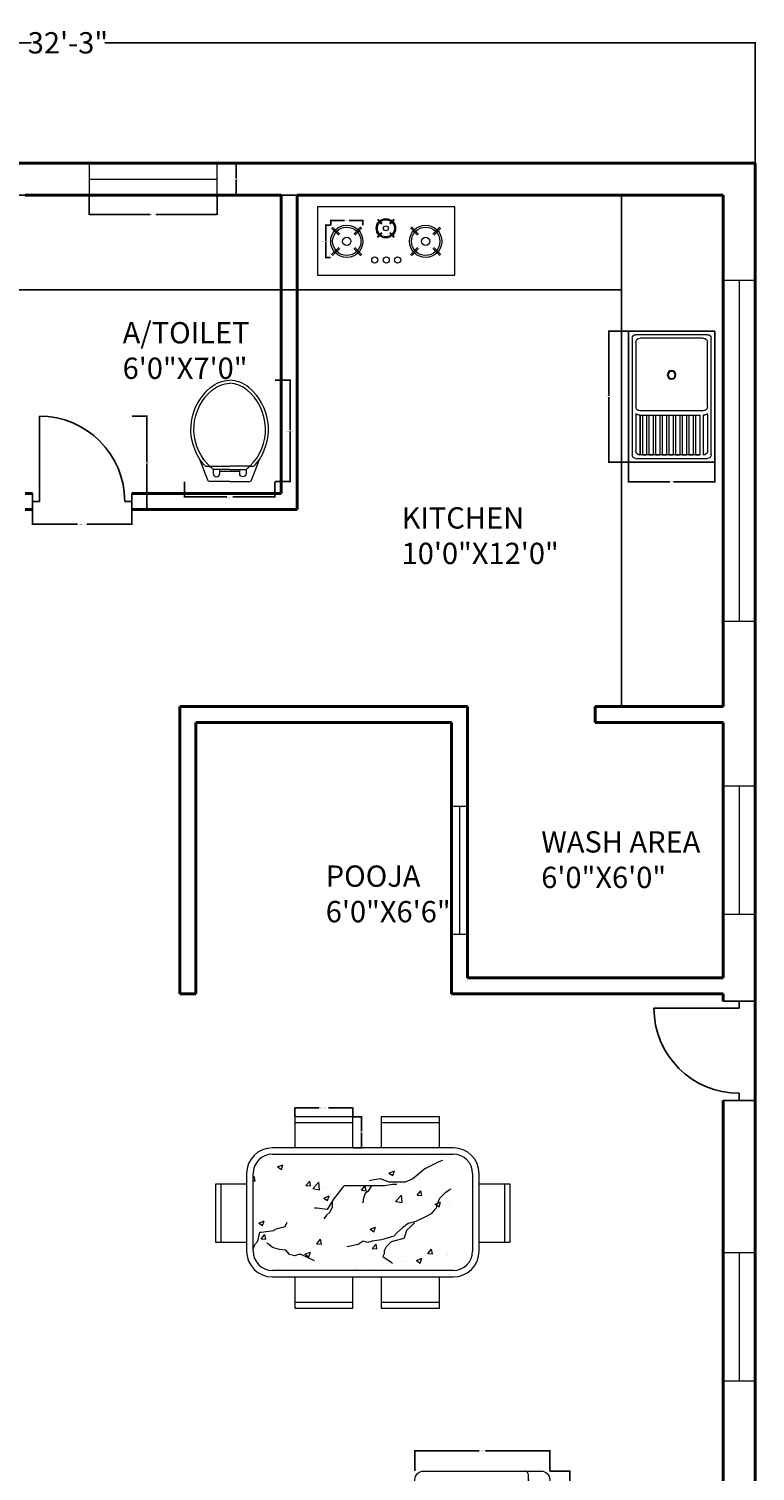
# Model space of a CAD drawing. Units: inches. Extents: x -19 to 419, y -828 to 43.
# Tile 9 of 9: x 205 to 410, y -364 to 43. Entities that reach past the tile are written whole.
import ezdxf

# ---------------------------------------------------------------- set-up
doc = ezdxf.new("R2010")
doc.units = ezdxf.units.IN
doc.header["$MEASUREMENT"] = 0
for name, color, linetype, lineweight in [('A-ANNO-DIMS', 2, 'Continuous', 18), ('A-AREA-IDEN', 7, 'Continuous', 25), ('A-DOOR', 3, 'Continuous', 25), ('A-EQPM', 9, 'Continuous', 20), ('A-FLOR-CASE', 8, 'Continuous', 25), ('A-FLOR-FIXT', 9, 'Continuous', 20), ('A-FURN', 8, 'Continuous', 18), ('A-FURN-PATT', 252, 'Continuous', 13), ('A-GLAZ', 4, 'Continuous', 20), ('A-WALL', 7, 'Continuous', 40)]:
    doc.layers.add(name, color=color, linetype=linetype, lineweight=lineweight)
doc.styles.get("Standard").update_dxf_attribs({"font": 'arial.ttf'})
doc.dimstyles.get("Standard").update_dxf_attribs({"dimtxt": 0.18, "dimasz": 0.18, "dimexe": 0.18, "dimexo": 0.0625, "dimgap": 0.09, "dimtad": 0, "dimtih": 1, "dimtoh": 1, "dimdec": 0, "dimzin": 0, "dimdsep": 46, "dimlunit": 3, "dimtxsty": 'Standard', "dimcen": 0.09, "dimadec": 0, "dimazin": 0, "dimtfac": 1, "dimtdec": 0, "dimtofl": 0, "dimtmove": 0, "dimatfit": 3, "dimfxl": 1, "dimtolj": 1, "dimtzin": 0, "dimarcsym": 0})

# ---------------------------------------------------------------- blocks, each defined once
blk = doc.blocks.new('*D1')
at = {"layer": 'A-ANNO-DIMS', "color": 0, "lineweight": -2, "transparency": 16777216}
for p, q in [((22.74, 4.83), (22.74, 38.87)), ((22.92, 38.69), (205.85, 38.69)), ((409.56, 38.69), (226.63, 38.69)), ((409.74, 4.83), (409.74, 38.87))]:
    blk.add_line(p, q, dxfattribs=at)
at = {"layer": 'A-ANNO-DIMS', "color": 0, "transparency": 16777216}
for points in [[(22.92, 38.72), (22.92, 38.66), (22.74, 38.69)], [(409.56, 38.72), (409.56, 38.66), (409.74, 38.69)]]:
    blk.add_solid(points, dxfattribs=at)
at = {"layer": 'Defpoints', "color": 0, "transparency": 16777216}
for p in [(409.74, 38.69), (22.74, 4.77), (409.74, 4.77)]:
    blk.add_point(p, dxfattribs=at)
at = {"layer": 'A-ANNO-DIMS', "color": 0, "transparency": 16777216, "insert": (216.24, 38.69), "char_height": 6, "attachment_point": 5}
blk.add_mtext('\\A1;32\'-3"', dxfattribs=at)
blk = doc.blocks.new('М12 540х820')
for p, q in [((0, 540), (-820, 540)), ((-820, 540), (-820, 0)), ((-797.5, 495), (-797.5, 45)), ((-45, 517.5), (-775, 517.5)), ((-775, 468), (-775, 72)), ((-347.5, 495), (-748, 495)), ((-320.5, 468), (-320.5, 72)), ((-301.7, 495), (-64.8, 495)), ((-293.7, 468), (-293.7, 472.5)), ((-293.7, 468), (-45, 468)), ((-45, 469.5), (-45, 468)), ((-22.5, 45), (-22.5, 495)), ((0, 0), (0, 540)), ((-293.7, 446.6), (-45, 446.6)), ((-293.7, 419.6), (-293.7, 446.6)), ((-293.7, 419.6), (-45, 419.6)), ((-293.7, 405), (-45, 405)), ((-293.7, 378), (-293.7, 405)), ((-293.7, 378), (-45, 378)), ((-293.7, 336.4), (-293.7, 363.4)), ((-293.7, 363.4), (-45, 363.4)), ((-45, 419.6), (-45, 446.6)), ((-45, 378), (-45, 405)), ((-45, 336.4), (-45, 363.4)), ((-293.7, 336.4), (-45, 336.4)), ((-293.7, 294.7), (-293.7, 321.7)), ((-293.7, 321.7), (-45, 321.7)), ((-293.7, 294.7), (-45, 294.7)), ((-293.7, 253.1), (-293.7, 280.1)), ((-293.7, 280.1), (-45, 280.1)), ((-45, 294.7), (-45, 321.7)), ((-45, 253.1), (-45, 280.1)), ((-293.7, 253.1), (-45, 253.1)), ((-293.7, 211.5), (-293.7, 238.5)), ((-293.7, 238.5), (-45, 238.5)), ((-293.7, 211.5), (-45, 211.5)), ((-293.7, 169.9), (-293.7, 196.9)), ((-293.7, 196.9), (-45, 196.9)), ((-45, 211.5), (-45, 238.5)), ((-45, 169.9), (-45, 196.9)), ((-293.7, 169.9), (-45, 169.9)), ((-293.7, 128.2), (-293.7, 155.2)), ((-293.7, 155.2), (-45, 155.2)), ((-293.7, 128.2), (-45, 128.2)), ((-293.7, 113.6), (-45, 113.6)), ((-293.7, 86.6), (-293.7, 113.6)), ((-45, 128.2), (-45, 155.2)), ((-45, 86.6), (-45, 113.6)), ((-820, 0), (0, 0)), ((-775, 22.5), (-45, 22.5)), ((-748, 45), (-347.5, 45)), ((-301.7, 45), (-64.8, 45)), ((-293.7, 86.6), (-45, 86.6)), ((-293.7, 72), (-45, 72)), ((-45, 70.5), (-45, 72))]:
    blk.add_line(p, q)
at = {"ltscale": 0.06}
for p, q in [((-820, 0), (-820, 540)), ((-820, 540), (0, 540)), ((0, 540), (0, 536.9)), ((0, 536.9), (0, 0)), ((-293.7, 446.6), (-45, 446.6)), ((-293.7, 405), (-293.7, 446.6)), ((-293.7, 363.4), (-293.7, 405)), ((-293.7, 321.7), (-293.7, 363.4)), ((-45, 446.6), (-45, 419.6)), ((-45, 419.6), (-45, 378)), ((-45, 378), (-45, 336.4)), ((-293.7, 280.1), (-293.7, 321.7)), ((-293.7, 238.5), (-293.7, 280.1)), ((-45, 336.4), (-45, 294.7)), ((-45, 294.7), (-45, 253.1)), ((-293.7, 196.9), (-293.7, 238.5)), ((-293.7, 155.2), (-293.7, 196.9)), ((-45, 253.1), (-45, 211.5)), ((-45, 211.5), (-45, 169.9)), ((-293.7, 113.6), (-293.7, 155.2)), ((-293.7, 72), (-293.7, 113.6)), ((-45, 169.9), (-45, 128.2)), ((-45, 128.2), (-45, 86.6)), ((0, 0), (-820, 0)), ((-45, 72), (-293.7, 72)), ((-45, 86.6), (-45, 72))]:
    blk.add_line(p, q, dxfattribs=at)
at = {"extrusion": (0, 0, -1)}
for centre, major_axis, start_param, end_param in [((-775, 495), (-15.9, 15.9), -0.785398, 0.785398), ((-775, 495), (-15.9, 15.9), -0.785398, 0.785398), ((-748, 468), (-19.1, -19.1), 0.785398, 2.356194), ((-748, 468), (-19.1, -19.1), 0.785398, 2.356194), ((-347.5, 468), (-19.1, 19.1), 0.785398, 2.356194), ((-347.5, 468), (-19.1, 19.1), 0.785398, 2.356194), ((-343.2, 468), (-35, 35), 1.779263, 2.356194), ((-343.2, 468), (-35, 35), 1.779263, 2.356192), ((-343.2, 468), (-35, 35), 2.356192, 2.356194), ((-72.3, 468.8), (-19.3, 19.3), 1.0328, 2.38382), ((-72.3, 468.8), (-19.3, 19.3), 1.0328, 1.064673), ((-72.3, 468.8), (-19.3, 19.3), 1.064673, 2.328569), ((-45, 495), (-15.9, -15.9), 2.356194, 3.926991), ((-45, 495), (-15.9, -15.9), 2.356194, 3.926991), ((-72.3, 468.8), (-19.3, 19.3), 2.328569, 2.38382), ((-545.5, 270), (-19.1, -19.1), 3.926991, 10.210176), ((-545.5, 270), (-19.1, -19.1), 3.926991, 10.210176), ((-545.5, 270), (-15.9, -15.9), 3.926991, 10.210176), ((-545.5, 270), (-15.9, -15.9), 3.926991, 10.210176), ((-775, 45), (-15.9, -15.9), 5.497787, 7.068583), ((-775, 45), (-15.9, -15.9), 5.497787, 7.068583), ((-748, 72), (-19.1, 19.1), 3.926991, 5.497787), ((-748, 72), (-19.1, 19.1), 3.926991, 5.497787), ((-347.5, 72), (-19.1, -19.1), 3.926991, 5.497787), ((-347.5, 72), (-19.1, -19.1), 3.926991, 5.497787), ((-343.2, 72), (-35, -35), 3.926991, 4.503922), ((-343.2, 72), (-35, -35), 3.926991, 4.503922), ((-72.3, 71.2), (-19.3, -19.3), 3.899365, 5.250385), ((-72.3, 71.2), (-19.3, -19.3), 5.218512, 5.250385), ((-72.3, 71.2), (-19.3, -19.3), 3.954617, 5.218512), ((-72.3, 71.2), (-19.3, -19.3), 3.899365, 3.954617), ((-45, 45), (-15.9, 15.9), 2.356194, 3.926991), ((-45, 45), (-15.9, 15.9), 2.356194, 3.926991)]:
    blk.add_ellipse(centre, major_axis=major_axis, ratio=1, start_param=start_param, end_param=end_param, dxfattribs=at)
blk = doc.blocks.new('DAY BED1')
at = {"color": 0}
blk.add_line((0.3, 0.25), (0.225, 0.255), dxfattribs=at)
blk.add_lwpolyline([(-0.3, 0, -0.414214), (-0.4, 0.1), (-0.4, 0.1, 0.317837), (-0.4, 0.1, -0.414214), (-0.4, 0.1), (-0.4, 0.1, 1.186185), (-0.4, 0.1, -0.414214), (-0.4, 0.1), (-0.4, 1.5, -0.414214), (-0.3, 1.6), (0.3, 1.6, -0.414214), (0.4, 1.5), (0.4, 0.1, -0.414214), (0.3, 0)], format="xyb", close=True, dxfattribs=at)
for points in [[(-0.073, 1.45), (-0.15, 1.45, -0.414214), (-0.2, 1.5), (-0.2, 1.55, -0.414214), (-0.15, 1.6)], [(-0.076, 1.425, -0.356772), (0.05, 1.568, -0.249542), (0.154, 1.438, 9.61688)], [(0.05, 1.568, -0.14773), (0.136, 1.422, -0.213343), (0.262, 1.293, -0.178662)], [(-0.073, 1.45, 0.165541), (-0.139, 1.419, 0.200231), (-0.058, 1.221, 0.121523)], [(0.143, 1.442, -0.306663), (0.262, 1.293, -0.30633), (0.154, 1.196, 0.872847)], [(0.25, 1.345), (0.25, 1.45), (0.152, 1.45, -0.414214)], [(0.2, 1.412), (0.2, 1.43, -0.414214), (0.22, 1.45), (0.23, 1.45, -0.414214), (0.25, 1.43)], [(0.25, 1.43), (0.25, 1.345, -0.414214)], [(-0.076, 1.156, -0.356772), (0.05, 1.299, -0.249542), (0.154, 1.169, 9.61688)], [(0.05, 1.299, -0.14773), (0.136, 1.153, -0.213343), (0.262, 1.024, -0.178662)], [(0.168, 1.163, 0.071865), (0.187, 1.205, -7.115464)], [(0.2, 1.142), (0.2, 1.211, -0.414214)], [(0.25, 1.262), (0.25, 1.075, -0.414214)], [(-0.073, 1.181, 0.165541), (-0.139, 1.15, 0.425989), (0.148, 0.869, 0.121523), (0.187, 0.936, -7.115464)], [(0.143, 1.173, -0.306663), (0.262, 1.024, -0.30633), (0.154, 0.926, 0.872847)], [(0.25, 0.992), (0.25, 0.275, -0.414214), (0.23, 0.255), (0.22, 0.255, -0.414214), (0.2, 0.275), (0.2, 0.942, -0.414214)], [(0.25, 0.377), (0.25, 0.3, 0.414214), (0.3, 0.25), (0.35, 0.25, 0.414214), (0.4, 0.3)]]:
    blk.add_lwpolyline(points, format="xyb", dxfattribs=at)
for points in [[(0.25, 1.075), (0.25, 1.262)], [(0.25, 0.377), (0.25, 0.992)]]:
    blk.add_lwpolyline(points, dxfattribs=at)
blk = doc.blocks.new('WIN-36X9')
for p, q in [((36, 9), (0, 9)), ((0, 9), (0, 0)), ((36, 0), (36, 9)), ((0, 4.5), (36, 4.5)), ((0, 0), (36, 0))]:
    blk.add_line(p, q)
blk = doc.blocks.new('WIN-96X9')
for p, q in [((96, 9), (0, 9)), ((0, 9), (0, 0)), ((96, 0), (96, 9)), ((0, 4.5), (96, 4.5)), ((0, 0), (96, 0))]:
    blk.add_line(p, q)
blk = doc.blocks.new('DOOR-24-PARTITION')
for p, q in [((2, 2.25), (2, 26.25)), ((0, 4.5), (0, 0)), ((28, 2.25), (28, 4.5)), ((0, 2.25), (2, 2.25)), ((26, 2.25), (28, 2.25)), ((28, 2.25), (28, 0))]:
    blk.add_line(p, q)
blk.add_arc((2, 2.25), 24, 0, 90)
blk = doc.blocks.new('DOOR-24-EXTERIOR')
for p, q in [((4.5, 28), (0, 28)), ((4.5, 26), (4.5, 28)), ((4.5, 28), (9, 28)), ((4.5, 0), (4.5, 2)), ((4.5, 2), (28.5, 2)), ((9, 0), (0, 0))]:
    blk.add_line(p, q)
blk.add_arc((4.5, 2), 24, 0, 90)
blk = doc.blocks.new('WC-FLOOR-MOUNT')
for p, q in [((4.1, 4.33), (5.3, 4.33)), ((5.3, 4.33), (10.92, 4.33)), ((16.55, 4.33), (10.92, 4.33)), ((16.55, 4.33), (17.75, 4.33))]:
    blk.add_line(p, q)
for points in [[(2.55, 6.29, -0.383919), (5.55, 26.53, -0.163732), (10.92, 28.59, -0.359733)], [(19.29, 6.29, 0.383919), (16.3, 26.53, 0.163732), (10.92, 28.59, 0.359733)], [(4.72, 4.91, -0.431639), (6.09, 25.87, -0.162618), (10.92, 27.73, -0.470877)], [(16.55, 4.33, 0.448546), (15.75, 25.87, 0.162618), (10.92, 27.73, 0.470877)], [(4.1, 4.33, -0.040937), (2.55, 6.29, -0.163732)], [(10.92, 0), (5.46, 0, -0.31031), (4.79, 0.46), (2.55, 6.29, -0.209071)], [(5.3, 4.33, -0.014165), (4.72, 4.91, -0.162618)], [(6.28, 3.47, -0.022712), (5.3, 4.33, -0.162618)], [(10.92, 0), (16.38, 0, 0.31031), (17.05, 0.46), (19.29, 6.29, 0.209071)], [(15.56, 3.47, 0.022712), (16.55, 4.33, 0.162618)], [(17.75, 4.33, 0.040937), (19.29, 6.29, 0.163732)], [(10.92, 3.47), (6.28, 3.47, -0.022712)], [(6.28, 3.47), (6.28, 2.27, 1), (8.11, 2.27), (8.11, 2.89)], [(10.92, 3.47), (15.56, 3.47, 0.476108)], [(15.56, 3.47), (15.56, 2.27, -1), (13.74, 2.27), (13.74, 2.89)]]:
    blk.add_lwpolyline(points, format="xyb")
for points in [[(8.11, 2.89), (8.11, 3.47)], [(13.74, 2.89), (8.11, 2.89)], [(13.74, 2.89), (13.74, 3.47)]]:
    blk.add_lwpolyline(points)
blk = doc.blocks.new('CHAIR-DINING')
for p, q in [((8.77, 16.37), (0, 16.37)), ((7.17, 16.37), (7.17, 0)), ((8.77, 0), (8.77, 16.37)), ((0, 0), (8.77, 0))]:
    blk.add_line(p, q)
blk = doc.blocks.new('COOKTOP-BURNER')
for p, q in [((2.27, 6.28), (0.26, 8.29)), ((2.54, 6.54), (0.52, 8.56)), ((6.53, 6.56), (8.52, 8.59)), ((6.8, 6.3), (8.79, 8.32)), ((2.27, 2.8), (0.26, 0.79)), ((2.54, 2.54), (0.52, 0.52)), ((6.53, 2.52), (8.52, 0.49)), ((6.8, 2.79), (8.79, 0.76))]:
    blk.add_line(p, q)
for radius in [4.54, 4, 1.17]:
    blk.add_circle((4.54, 4.54), radius)
blk = doc.blocks.new('*D16')
at = {"layer": 'A-ANNO-DIMS', "color": 0, "lineweight": -2, "transparency": 16777216}
for p, q in [((222.24, -4.3), (222.24, -9.81)), ((258.24, -4.3), (258.24, -9.81)), ((222.42, -9.63), (239.37, -9.63)), ((258.06, -9.63), (241.1, -9.63))]:
    blk.add_line(p, q, dxfattribs=at)
at = {"layer": 'A-ANNO-DIMS', "color": 0, "transparency": 16777216}
for points in [[(222.42, -9.6), (222.42, -9.66), (222.24, -9.63)], [(258.06, -9.6), (258.06, -9.66), (258.24, -9.63)]]:
    blk.add_solid(points, dxfattribs=at)
at = {"layer": 'Defpoints', "color": 0, "transparency": 16777216}
for p in [(222.24, -4.23), (258.24, -4.23), (258.24, -9.63)]:
    blk.add_point(p, dxfattribs=at)
at = {"layer": 'A-ANNO-DIMS', "color": 0, "transparency": 16777216, "insert": (240.24, -9.63), "char_height": 0.18, "attachment_point": 5}
blk.add_mtext('\\A1;W1 3\'-0" TYP.', dxfattribs=at)
blk = doc.blocks.new('*D17')
at = {"layer": 'A-ANNO-DIMS', "color": 0, "lineweight": -2, "transparency": 16777216}
for p, q in [((258.3, 4.77), (263.82, 4.77)), ((263.64, 4.59), (263.64, 0.45)), ((263.64, -4.05), (263.64, 0.08)), ((258.3, -4.23), (263.82, -4.23))]:
    blk.add_line(p, q, dxfattribs=at)
at = {"layer": 'A-ANNO-DIMS', "color": 0, "transparency": 16777216}
for points in [[(263.61, 4.59), (263.67, 4.59), (263.64, 4.77)], [(263.61, -4.05), (263.67, -4.05), (263.64, -4.23)]]:
    blk.add_solid(points, dxfattribs=at)
at = {"layer": 'Defpoints', "color": 0, "transparency": 16777216}
for p in [(258.24, 4.77), (263.64, 4.77), (258.24, -4.23)]:
    blk.add_point(p, dxfattribs=at)
at = {"layer": 'A-ANNO-DIMS', "color": 0, "transparency": 16777216, "insert": (263.64, 0.27), "char_height": 0.18, "attachment_point": 5}
blk.add_mtext('\\A1;0\'-9" TYP.', dxfattribs=at)
blk = doc.blocks.new('*D22')
at = {"layer": 'A-ANNO-DIMS', "color": 0, "lineweight": -2, "transparency": 16777216}
for p, q in [((206.24, -92.8), (206.24, -97.11)), ((234.24, -92.8), (234.24, -97.11)), ((206.42, -96.93), (218.92, -96.93)), ((234.06, -96.93), (221.56, -96.93))]:
    blk.add_line(p, q, dxfattribs=at)
at = {"layer": 'A-ANNO-DIMS', "color": 0, "transparency": 16777216}
for points in [[(206.42, -96.9), (206.42, -96.96), (206.24, -96.93)], [(234.06, -96.9), (234.06, -96.96), (234.24, -96.93)]]:
    blk.add_solid(points, dxfattribs=at)
at = {"layer": 'Defpoints', "color": 0, "transparency": 16777216}
for p in [(206.24, -92.73), (234.24, -92.73), (234.24, -96.93)]:
    blk.add_point(p, dxfattribs=at)
at = {"layer": 'A-ANNO-DIMS', "color": 0, "transparency": 16777216, "insert": (220.24, -96.93), "char_height": 0.18, "attachment_point": 5}
blk.add_mtext('\\A1;INT. DOOR 2\'-4" TYP.', dxfattribs=at)
blk = doc.blocks.new('*D23')
at = {"layer": 'A-ANNO-DIMS', "color": 0, "lineweight": -2, "transparency": 16777216}
for p, q in [((234.3, -66.48), (238.62, -66.48)), ((238.44, -66.66), (238.44, -79.43)), ((238.44, -92.55), (238.44, -79.79)), ((234.3, -92.73), (238.62, -92.73))]:
    blk.add_line(p, q, dxfattribs=at)
at = {"layer": 'A-ANNO-DIMS', "color": 0, "transparency": 16777216}
for points in [[(238.41, -66.66), (238.47, -66.66), (238.44, -66.48)], [(238.41, -92.55), (238.47, -92.55), (238.44, -92.73)]]:
    blk.add_solid(points, dxfattribs=at)
at = {"layer": 'Defpoints', "color": 0, "transparency": 16777216}
for p in [(234.24, -66.48), (238.44, -66.48), (234.24, -92.73)]:
    blk.add_point(p, dxfattribs=at)
at = {"layer": 'A-ANNO-DIMS', "color": 0, "transparency": 16777216, "insert": (238.44, -79.61), "char_height": 0.18, "attachment_point": 5}
blk.add_mtext('\\A1;2\'-2 1/2" TYP.', dxfattribs=at)
blk = doc.blocks.new('*D28')
at = {"layer": 'A-ANNO-DIMS', "color": 0, "lineweight": -2, "transparency": 16777216}
for p, q in [((280.11, -263.75), (280.11, -261.18)), ((280.29, -261.36), (287.02, -261.36)), ((296.3, -261.36), (289.57, -261.36)), ((296.48, -263.75), (296.48, -261.18))]:
    blk.add_line(p, q, dxfattribs=at)
at = {"layer": 'A-ANNO-DIMS', "color": 0, "transparency": 16777216}
for points in [[(280.29, -261.33), (280.29, -261.39), (280.11, -261.36)], [(296.3, -261.33), (296.3, -261.39), (296.48, -261.36)]]:
    blk.add_solid(points, dxfattribs=at)
at = {"layer": 'Defpoints', "color": 0, "transparency": 16777216}
for p in [(280.11, -261.36), (280.11, -263.81), (296.48, -263.81)]:
    blk.add_point(p, dxfattribs=at)
at = {"layer": 'A-ANNO-DIMS', "color": 0, "transparency": 16777216, "insert": (288.3, -261.36), "char_height": 0.18, "attachment_point": 5}
blk.add_mtext('\\A1;CHAIR 1\'-4 1/2" TYP.', dxfattribs=at)
blk = doc.blocks.new('*D29')
at = {"layer": 'A-ANNO-DIMS', "color": 0, "lineweight": -2, "transparency": 16777216}
for p, q in [((296.54, -263.81), (299.12, -263.81)), ((298.94, -263.99), (298.94, -268.01)), ((298.94, -272.4), (298.94, -268.38)), ((296.54, -272.58), (299.12, -272.58))]:
    blk.add_line(p, q, dxfattribs=at)
at = {"layer": 'A-ANNO-DIMS', "color": 0, "transparency": 16777216}
for points in [[(298.91, -263.99), (298.97, -263.99), (298.94, -263.81)], [(298.91, -272.4), (298.97, -272.4), (298.94, -272.58)]]:
    blk.add_solid(points, dxfattribs=at)
at = {"layer": 'Defpoints', "color": 0, "transparency": 16777216}
for p in [(296.48, -263.81), (298.94, -263.81), (296.48, -272.58)]:
    blk.add_point(p, dxfattribs=at)
at = {"layer": 'A-ANNO-DIMS', "color": 0, "transparency": 16777216, "insert": (298.94, -268.19), "char_height": 0.18, "attachment_point": 5}
blk.add_mtext('\\A1;0\'-9" TYP.', dxfattribs=at)
blk = doc.blocks.new('*D34')
at = {"layer": 'A-ANNO-DIMS', "color": 0, "lineweight": -2, "transparency": 16777216}
for p, q in [((274.56, -56.34), (278.96, -56.34)), ((278.78, -56.52), (278.78, -70.45)), ((278.78, -84.75), (278.78, -70.82)), ((274.56, -84.93), (278.96, -84.93))]:
    blk.add_line(p, q, dxfattribs=at)
at = {"layer": 'A-ANNO-DIMS', "color": 0, "transparency": 16777216}
for points in [[(278.75, -56.52), (278.81, -56.52), (278.78, -56.34)], [(278.75, -84.75), (278.81, -84.75), (278.78, -84.93)]]:
    blk.add_solid(points, dxfattribs=at)
at = {"layer": 'Defpoints', "color": 0, "transparency": 16777216}
for p in [(274.49, -56.34), (278.78, -56.34), (274.49, -84.93)]:
    blk.add_point(p, dxfattribs=at)
at = {"layer": 'A-ANNO-DIMS', "color": 0, "transparency": 16777216, "insert": (278.78, -70.63), "char_height": 0.18, "attachment_point": 5}
blk.add_mtext('\\A1;WC 2\'-4 1/2" TYP.', dxfattribs=at)
blk = doc.blocks.new('*D35')
at = {"layer": 'A-ANNO-DIMS', "color": 0, "lineweight": -2, "transparency": 16777216}
for p, q in [((249.1, -84.99), (249.1, -89.4)), ((274.49, -84.99), (274.49, -89.4)), ((249.28, -89.22), (260.95, -89.22)), ((274.31, -89.22), (262.65, -89.22))]:
    blk.add_line(p, q, dxfattribs=at)
at = {"layer": 'A-ANNO-DIMS', "color": 0, "transparency": 16777216}
for points in [[(249.28, -89.19), (249.28, -89.25), (249.1, -89.22)], [(274.31, -89.19), (274.31, -89.25), (274.49, -89.22)]]:
    blk.add_solid(points, dxfattribs=at)
at = {"layer": 'Defpoints', "color": 0, "transparency": 16777216}
for p in [(249.1, -84.93), (274.49, -84.93), (274.49, -89.22)]:
    blk.add_point(p, dxfattribs=at)
at = {"layer": 'A-ANNO-DIMS', "color": 0, "transparency": 16777216, "insert": (261.8, -89.22), "char_height": 0.18, "attachment_point": 5}
blk.add_mtext('\\A1;2\'-1 1/2" TYP.', dxfattribs=at)
blk = doc.blocks.new('*D36')
at = {"layer": 'A-ANNO-DIMS', "color": 0, "lineweight": -2, "transparency": 16777216}
for p, q in [((290.16, -12.69), (288.68, -12.69)), ((288.86, -12.87), (288.86, -17.05)), ((288.86, -21.59), (288.86, -17.41)), ((290.16, -21.77), (288.68, -21.77))]:
    blk.add_line(p, q, dxfattribs=at)
at = {"layer": 'A-ANNO-DIMS', "color": 0, "transparency": 16777216}
for points in [[(288.83, -12.87), (288.89, -12.87), (288.86, -12.69)], [(288.83, -21.59), (288.89, -21.59), (288.86, -21.77)]]:
    blk.add_solid(points, dxfattribs=at)
at = {"layer": 'Defpoints', "color": 0, "transparency": 16777216}
for p in [(288.86, -12.69), (290.22, -12.69), (290.22, -21.77)]:
    blk.add_point(p, dxfattribs=at)
at = {"layer": 'A-ANNO-DIMS', "color": 0, "transparency": 16777216, "insert": (288.86, -17.23), "char_height": 0.18, "attachment_point": 5}
blk.add_mtext('\\A1;BURNER 0\'-9" TYP.', dxfattribs=at)
blk = doc.blocks.new('*D37')
at = {"layer": 'A-ANNO-DIMS', "color": 0, "lineweight": -2, "transparency": 16777216}
for p, q in [((290.22, -12.63), (290.22, -11.15)), ((290.4, -11.33), (294.12, -11.33)), ((299.12, -11.33), (295.4, -11.33)), ((299.3, -12.63), (299.3, -11.15))]:
    blk.add_line(p, q, dxfattribs=at)
at = {"layer": 'A-ANNO-DIMS', "color": 0, "transparency": 16777216}
for points in [[(290.4, -11.3), (290.4, -11.36), (290.22, -11.33)], [(299.12, -11.3), (299.12, -11.36), (299.3, -11.33)]]:
    blk.add_solid(points, dxfattribs=at)
at = {"layer": 'Defpoints', "color": 0, "transparency": 16777216}
for p in [(299.3, -11.33), (290.22, -12.69), (299.3, -12.69)]:
    blk.add_point(p, dxfattribs=at)
at = {"layer": 'A-ANNO-DIMS', "color": 0, "transparency": 16777216, "insert": (294.76, -11.33), "char_height": 0.18, "attachment_point": 5}
blk.add_mtext('\\A1;0\'-9" TYP.', dxfattribs=at)
blk = doc.blocks.new('*D40')
at = {"layer": 'A-ANNO-DIMS', "color": 0, "lineweight": -2, "transparency": 16777216}
for p, q in [((374.02, -42.51), (368.36, -42.51)), ((368.54, -42.69), (368.54, -60.77)), ((368.54, -79.23), (368.54, -61.14)), ((374.02, -79.41), (368.36, -79.41))]:
    blk.add_line(p, q, dxfattribs=at)
at = {"layer": 'A-ANNO-DIMS', "color": 0, "transparency": 16777216}
for points in [[(368.51, -42.69), (368.57, -42.69), (368.54, -42.51)], [(368.51, -79.23), (368.57, -79.23), (368.54, -79.41)]]:
    blk.add_solid(points, dxfattribs=at)
at = {"layer": 'Defpoints', "color": 0, "transparency": 16777216}
for p in [(374.08, -42.51), (368.54, -79.41), (374.08, -79.41)]:
    blk.add_point(p, dxfattribs=at)
at = {"layer": 'A-ANNO-DIMS', "color": 0, "transparency": 16777216, "insert": (368.54, -60.96), "char_height": 0.18, "attachment_point": 5}
blk.add_mtext('\\A1;SINK 3\'-1"', dxfattribs=at)
blk = doc.blocks.new('*D41')
at = {"layer": 'A-ANNO-DIMS', "color": 0, "lineweight": -2, "transparency": 16777216}
for p, q in [((374.08, -79.47), (374.08, -85.12)), ((398.38, -79.47), (398.38, -85.12)), ((374.26, -84.94), (385.69, -84.94)), ((398.2, -84.94), (386.77, -84.94))]:
    blk.add_line(p, q, dxfattribs=at)
at = {"layer": 'A-ANNO-DIMS', "color": 0, "transparency": 16777216}
for points in [[(374.26, -84.91), (374.26, -84.97), (374.08, -84.94)], [(398.2, -84.91), (398.2, -84.97), (398.38, -84.94)]]:
    blk.add_solid(points, dxfattribs=at)
at = {"layer": 'Defpoints', "color": 0, "transparency": 16777216}
for p in [(374.08, -79.41), (398.38, -79.41), (398.38, -84.94)]:
    blk.add_point(p, dxfattribs=at)
at = {"layer": 'A-ANNO-DIMS', "color": 0, "transparency": 16777216, "insert": (386.23, -84.94), "char_height": 0.18, "attachment_point": 5}
blk.add_mtext('\\A1;2\'-0 1/2"', dxfattribs=at)
blk = doc.blocks.new('*D42')
at = {"layer": 'A-ANNO-DIMS', "color": 0, "lineweight": -2, "transparency": 16777216}
for p, q in [((313.95, -363.6), (313.95, -357.79)), ((314.13, -357.97), (332.01, -357.97)), ((351.71, -357.97), (333.83, -357.97)), ((351.89, -363.6), (351.89, -357.79))]:
    blk.add_line(p, q, dxfattribs=at)
at = {"layer": 'A-ANNO-DIMS', "color": 0, "transparency": 16777216}
for points in [[(314.13, -357.94), (314.13, -358), (313.95, -357.97)], [(351.71, -357.94), (351.71, -358), (351.89, -357.97)]]:
    blk.add_solid(points, dxfattribs=at)
at = {"layer": 'Defpoints', "color": 0, "transparency": 16777216}
for p in [(313.95, -357.97), (313.95, -363.66), (351.89, -363.66)]:
    blk.add_point(p, dxfattribs=at)
at = {"layer": 'A-ANNO-DIMS', "color": 0, "transparency": 16777216, "insert": (332.92, -357.97), "char_height": 0.18, "attachment_point": 5}
blk.add_mtext('\\A1;DAY BED 3\'-2"', dxfattribs=at)
blk = doc.blocks.new('*D43')
at = {"layer": 'A-ANNO-DIMS', "color": 0, "lineweight": -2, "transparency": 16777216}
for p, q in [((351.95, -363.66), (357.76, -363.66)), ((357.58, -363.84), (357.58, -372.97)), ((357.58, -382.45), (357.58, -373.33)), ((351.95, -382.63), (357.76, -382.63))]:
    blk.add_line(p, q, dxfattribs=at)
at = {"layer": 'A-ANNO-DIMS', "color": 0, "transparency": 16777216}
for points in [[(357.55, -363.84), (357.61, -363.84), (357.58, -363.66)], [(357.55, -382.45), (357.61, -382.45), (357.58, -382.63)]]:
    blk.add_solid(points, dxfattribs=at)
at = {"layer": 'Defpoints', "color": 0, "transparency": 16777216}
for p in [(351.89, -363.66), (357.58, -363.66), (351.89, -382.63)]:
    blk.add_point(p, dxfattribs=at)
at = {"layer": 'A-ANNO-DIMS', "color": 0, "transparency": 16777216, "insert": (357.58, -373.15), "char_height": 0.18, "attachment_point": 5}
blk.add_mtext('\\A1;1\'-7"', dxfattribs=at)
blk = doc.blocks.new('*D47')
at = {"layer": 'A-ANNO-DIMS', "color": 0, "lineweight": -2, "transparency": 16777216}
for p, q in [((372.05, -4.23), (-19.04, -4.23)), ((-18.86, -4.41), (-18.86, -17.36)), ((-18.86, -30.67), (-18.86, -17.72)), ((372.05, -30.85), (-19.04, -30.85))]:
    blk.add_line(p, q, dxfattribs=at)
at = {"layer": 'A-ANNO-DIMS', "color": 0, "transparency": 16777216}
for points in [[(-18.89, -4.41), (-18.83, -4.41), (-18.86, -4.23)], [(-18.89, -30.67), (-18.83, -30.67), (-18.86, -30.85)]]:
    blk.add_solid(points, dxfattribs=at)
at = {"layer": 'Defpoints', "color": 0, "transparency": 16777216}
for p in [(-18.86, -4.23), (372.11, -4.23), (372.11, -30.85)]:
    blk.add_point(p, dxfattribs=at)
at = {"layer": 'A-ANNO-DIMS', "color": 0, "transparency": 16777216, "insert": (-18.86, -17.54), "char_height": 0.18, "attachment_point": 5}
blk.add_mtext('\\A1;2\'-2 1/2"', dxfattribs=at)

msp = doc.modelspace()

# ---------------------------------------------------------------- hatches: boundary and pattern name
at = {"layer": 'A-FURN-PATT'}
h = msp.add_hatch(dxfattribs=at)
h.set_pattern_fill('AR-CONC', color=256, scale=2.1824, style=0)
h.paths.add_polyline_path([(268.36, -301.68), (268.38, -302.03), (268.41, -302.39), (268.47, -302.74), (268.55, -303.09), (268.65, -303.43), (268.78, -303.76), (268.93, -304.09), (269.09, -304.4), (269.28, -304.71), (269.49, -305), (269.72, -305.27), (269.96, -305.53), (270.22, -305.78), (270.5, -306), (270.79, -306.21), (271.09, -306.4), (271.41, -306.57), (271.73, -306.72), (272.07, -306.84), (272.41, -306.95), (272.76, -307.03), (273.11, -307.08), (273.46, -307.12), (273.82, -307.13), (324.74, -307.13), (325.1, -307.12), (325.45, -307.08), (325.81, -307.03), (326.15, -306.95), (326.5, -306.84), (326.83, -306.72), (327.16, -306.57), (327.47, -306.4), (327.77, -306.21), (328.06, -306), (328.34, -305.78), (328.6, -305.53), (328.84, -305.27), (329.07, -305), (329.28, -304.71), (329.47, -304.4), (329.64, -304.09), (329.78, -303.76), (329.91, -303.43), (330.01, -303.09), (330.09, -302.74), (330.15, -302.39), (330.19, -302.03), (330.2, -301.68), (330.2, -279.85), (330.19, -279.49), (330.15, -279.14), (330.09, -278.79), (330.01, -278.44), (329.91, -278.1), (329.78, -277.76), (329.64, -277.44), (329.47, -277.12), (329.28, -276.82), (329.07, -276.53), (328.84, -276.25), (328.6, -275.99), (328.34, -275.75), (328.06, -275.52), (327.77, -275.32), (327.47, -275.13), (327.16, -274.96), (326.83, -274.81), (326.5, -274.69), (326.15, -274.58), (325.81, -274.5), (325.45, -274.44), (325.1, -274.41), (324.74, -274.4), (273.82, -274.4), (273.46, -274.41), (273.11, -274.44), (272.76, -274.5), (272.41, -274.58), (272.07, -274.69), (271.73, -274.81), (271.41, -274.96), (271.09, -275.13), (270.79, -275.32), (270.5, -275.52), (270.22, -275.75), (269.96, -275.99), (269.72, -276.25), (269.49, -276.53), (269.28, -276.82), (269.09, -277.12), (268.93, -277.44), (268.78, -277.76), (268.65, -278.1), (268.55, -278.44), (268.47, -278.79), (268.41, -279.14), (268.38, -279.49), (268.36, -279.85)])

# ---------------------------------------------------------------- linework, layer by layer
at = {"layer": 'A-EQPM'}
for p, q in [((325.19, -7.47), (286.54, -7.47)), ((286.54, -7.47), (286.54, -26.8)), ((325.19, -26.8), (325.19, -7.47)), ((304.57, -12.36), (303.36, -11.15)), ((304.73, -12.2), (303.52, -10.99)), ((306.81, -12.2), (308.02, -10.99)), ((306.97, -12.36), (308.18, -11.15)), ((304.56, -14.75), (303.34, -15.95)), ((304.71, -14.91), (303.5, -16.11)), ((306.82, -14.91), (308.04, -16.11)), ((306.98, -14.75), (308.2, -15.95)), ((286.54, -26.8), (325.19, -26.8))]:
    msp.add_line(p, q, dxfattribs=at)
for centre, radius in [((305.77, -13.56), 2.72), ((305.77, -13.56), 2.4), ((305.77, -13.56), 0.702), ((302.64, -22.5), 0.859), ((305.86, -22.5), 0.859), ((309.08, -22.5), 0.859)]:
    msp.add_circle(centre, radius, dxfattribs=at)
at = {"layer": 'A-FLOR-CASE'}
for p, q in [((372.11, -30.85), (372.11, -4.23)), ((280.74, -30.85), (372.11, -30.85)), ((372.11, -30.85), (372.11, -148.23))]:
    msp.add_line(p, q, dxfattribs=at)
at = {"layer": 'A-FURN'}
for p, q in [((324.74, -272.58), (273.82, -272.58)), ((273.82, -274.4), (324.74, -274.4)), ((321.7, -276.16), (320.71, -276.55)), ((266.55, -279.85), (266.55, -301.68)), ((268.36, -301.68), (268.36, -279.85)), ((316.75, -278.53), (313.39, -281.29)), ((320.71, -276.55), (316.75, -278.53)), ((330.2, -279.85), (330.2, -301.68)), ((332.02, -301.68), (332.02, -279.85)), ((293.62, -283.66), (291.04, -287.02)), ((294.01, -283.27), (293.62, -283.66)), ((305.48, -283.27), (294.01, -283.27)), ((301.33, -283.85), (300.74, -284.84)), ((301.92, -281.69), (301.13, -281.88)), ((301.73, -283.26), (301.33, -283.85)), ((304.29, -281.29), (301.92, -281.69)), ((306.67, -282.28), (304.29, -281.29)), ((307.66, -282.87), (305.48, -283.27)), ((311.22, -282.28), (306.67, -282.28)), ((308.84, -282.87), (307.66, -282.87)), ((313.39, -281.29), (311.22, -282.28)), ((324.07, -284.25), (322.49, -285.24)), ((291.04, -287.02), (289.27, -289.98)), ((290.65, -287.61), (290.65, -289.39)), ((299.35, -287.6), (299.16, -288.2)), ((299.55, -286.42), (299.35, -287.21)), ((299.35, -287.21), (299.35, -287.6)), ((299.95, -285.43), (299.55, -286.42)), ((300.74, -284.84), (299.95, -285.43)), ((320.91, -286.82), (320.11, -288.6)), ((322.49, -285.24), (320.91, -286.82)), ((286.3, -289.59), (285.71, -289.59)), ((289.27, -289.98), (286.3, -289.59)), ((289.07, -291.56), (288.28, -292.55)), ((289.86, -290.77), (289.07, -291.56)), ((290.65, -289.39), (289.86, -290.77)), ((317.15, -291.96), (314.18, -293.34)), ((318.53, -291.17), (317.15, -291.96)), ((319.32, -290.18), (318.53, -291.17)), ((319.92, -289.59), (319.32, -290.18)), ((320.11, -288.6), (319.92, -289.59)), ((269.69, -298.87), (270.28, -296.3)), ((270.28, -296.3), (270.68, -296.3)), ((270.68, -296.3), (274.24, -295.91)), ((274.24, -295.91), (274.63, -295.51)), ((274.63, -295.51), (277.4, -294.72)), ((277.4, -294.72), (277.99, -293.54)), ((308.84, -296.5), (308.05, -297.49)), ((310.42, -295.12), (308.84, -296.5)), ((312.01, -293.93), (310.42, -295.12)), ((311.61, -295.91), (311.02, -297.69)), ((313, -294.53), (311.61, -295.91)), ((314.18, -293.34), (312.01, -293.93)), ((313.79, -293.74), (313, -294.53)), ((268.5, -300.85), (268.9, -299.86)), ((268.9, -299.86), (269.69, -298.87)), ((272.85, -299.85), (272.26, -299.46)), ((273.84, -300.64), (272.85, -299.85)), ((275.82, -301.23), (273.84, -300.64)), ((297.97, -299.86), (294.8, -300.45)), ((299.35, -298.87), (297.97, -299.86)), ((300.73, -299.27), (299.35, -298.87)), ((301.92, -298.87), (300.73, -299.27)), ((304.49, -298.48), (301.92, -298.87)), ((308.05, -297.49), (304.49, -298.48)), ((305.88, -300.45), (305.28, -301.64)), ((307.26, -299.07), (305.88, -300.45)), ((310.82, -298.08), (307.26, -299.07)), ((311.02, -297.69), (310.82, -298.08)), ((277.6, -301.43), (275.82, -301.23)), ((278.59, -302.62), (277.6, -301.43)), ((280.17, -303.01), (278.59, -302.62)), ((281.16, -302.62), (280.17, -303.01)), ((281.95, -302.62), (281.16, -302.62)), ((285.71, -304.39), (281.95, -302.62)), ((305.28, -302.43), (304.89, -303.22)), ((304.89, -303.22), (307.26, -304.8)), ((305.28, -301.64), (305.28, -302.43)), ((324.74, -307.13), (273.82, -307.13)), ((307.26, -304.8), (307.66, -305.19)), ((273.82, -308.95), (324.74, -308.95))]:
    msp.add_line(p, q, dxfattribs=at)
for centre, radius, start, end in [((273.82, -279.85), 7.27, 90, 180), ((273.82, -279.85), 5.46, 90, 180), ((324.74, -279.85), 7.27, 0, 90), ((324.74, -279.85), 5.46, 0, 90), ((273.82, -301.68), 7.27, 180, 270), ((273.82, -301.68), 5.46, 180, 270), ((324.74, -301.68), 5.46, 270, 0), ((324.74, -301.68), 7.27, 270, 0)]:
    msp.add_arc(centre, radius, start, end, dxfattribs=at)
at = {"layer": 'A-GLAZ'}
for p, q in [((324.24, -176.39), (324.24, -212.39)), ((328.74, -176.39), (324.24, -176.39)), ((326.49, -176.39), (326.49, -212.39)), ((328.74, -176.39), (328.74, -212.39)), ((324.24, -212.39), (328.74, -212.39))]:
    msp.add_line(p, q, dxfattribs=at)
at = {"layer": 'A-WALL'}
for p, q in [((22.74, 4.77), (409.74, 4.77)), ((409.74, 4.77), (409.74, -231.23)), ((204.24, -4.23), (276.24, -4.23)), ((276.24, -4.23), (276.24, -88.23)), ((280.74, -4.23), (280.74, -92.73)), ((280.74, -4.23), (400.74, -4.23)), ((400.74, -4.23), (400.74, -148.23)), ((204.24, -88.23), (206.24, -88.23)), ((234.24, -88.23), (276.24, -88.23)), ((204.24, -92.73), (206.24, -92.73)), ((234.24, -92.73), (280.74, -92.73)), ((247.74, -148.23), (328.74, -148.23)), ((247.74, -148.23), (247.74, -229.23)), ((328.74, -152.73), (328.74, -148.23)), ((364.74, -148.23), (364.74, -152.73)), ((364.74, -148.23), (400.74, -148.23)), ((252.24, -152.73), (324.24, -152.73)), ((252.24, -152.73), (252.24, -229.23)), ((324.24, -152.73), (324.24, -229.23)), ((328.74, -152.73), (328.74, -224.73)), ((364.74, -152.73), (400.74, -152.73)), ((400.74, -152.73), (400.74, -224.73)), ((328.74, -224.73), (400.74, -224.73)), ((247.74, -229.23), (252.24, -229.23)), ((324.24, -229.23), (400.74, -229.23)), ((400.74, -229.23), (400.74, -231.23)), ((409.74, -231.23), (409.74, -259.23)), ((400.74, -259.23), (400.74, -445.23)), ((409.74, -259.23), (409.74, -785.73))]:
    msp.add_line(p, q, dxfattribs=at)

# ---------------------------------------------------------------- block references
at = {"layer": 'A-DOOR'}
msp.add_blockref('DOOR-24-PARTITION', (206.24, -92.73), dxfattribs=at)
at = {"layer": 'A-DOOR', "rotation": 180}
msp.add_blockref('DOOR-24-EXTERIOR', (409.74, -231.23), dxfattribs=at)
at = {"layer": 'A-EQPM'}
msp.add_blockref('COOKTOP-BURNER', (290.22, -21.77), dxfattribs=at)
at = {"layer": 'A-EQPM', "rotation": 180}
msp.add_blockref('COOKTOP-BURNER', (321.5, -12.69), dxfattribs=at)
at = {"layer": 'A-FLOR-FIXT', "xscale": 0.0450002963905297, "yscale": 0.0450002963905297, "zscale": 0.0450002963905297, "rotation": 270}
msp.add_blockref('М12 540х820', (374.08, -79.41), dxfattribs=at)
at = {"layer": 'A-FLOR-FIXT'}
msp.add_blockref('WC-FLOOR-MOUNT', (250.87, -84.93), dxfattribs=at)
at = {"layer": 'A-FURN'}
for p, rotation in [((296.48, -272.58), 89.99999998729112), ((320.85, -272.58), 89.99999998729112), ((266.54, -282.8), 180), ((280.11, -308.95), 269.9999999884718), ((304.48, -308.95), 269.9999999884719)]:
    msp.add_blockref('CHAIR-DINING', p, dxfattribs=dict(at, rotation=rotation))
msp.add_blockref('CHAIR-DINING', (332.02, -299.17), dxfattribs=at)
at = {"layer": 'A-FURN', "ltscale": 0.03, "xscale": 23.71147996292152, "yscale": 23.71147996292152, "zscale": 23.71147996292152, "rotation": 90}
msp.add_blockref('DAY BED1', (351.89, -373.15), dxfattribs=at)
at = {"layer": 'A-GLAZ'}
msp.add_blockref('WIN-36X9', (222.24, -4.23), dxfattribs=at)
for name, p, rotation in [('WIN-96X9', (400.74, -28.23), 270.0000000000003), ('WIN-36X9', (400.74, -170.73), 270.0000000000001), ('WIN-36X9', (400.74, -302.18), 270.0000000000001)]:
    msp.add_blockref(name, p, dxfattribs=dict(at, rotation=rotation))

# ---------------------------------------------------------------- texts
at = {"layer": 'A-AREA-IDEN', "char_height": 6, "attachment_point": 1}
for s, insert in [('A/TOILET\\P6\'0"X7\'0"', (231.64, -39.99)), ('KITCHEN\\P10\'0"X12\'0"', (310.19, -92.14)), ('WASH AREA\\P6\'0"X6\'0"', (349.51, -183.41)), ('POOJA\\P6\'0"X6\'6"', (288.83, -193.05))]:
    msp.add_mtext(s, dxfattribs=dict(at, insert=insert))

# ---------------------------------------------------------------- dimensions: what is measured, and where the dimension line sits
at = {"layer": 'A-ANNO-DIMS'}
for base, p1, p2, override, picture, middle in [((409.74, 38.69), (22.74, 4.77), (409.74, 4.77), {"dimtxt": 6, "dimclrd": 0, "dimclre": 0, "dimclrt": 0}, '*D1', (216.24, 38.69)), ((398.38, -84.94), (374.08, -79.41), (398.38, -79.41), {"dimdec": 1, "dimlfac": 1, "dimrnd": 0, "dimzin": 1, "dimdsep": 46, "dimlunit": 4, "dimfrac": 2}, '*D41', (386.23, -84.94))]:
    dim = msp.add_linear_dim(base=base, p1=p1, p2=p2, dimstyle='Standard', override=override, dxfattribs=at)
    dim.commit()
    dim.dimension.update_dxf_attribs({"geometry": picture, "text_midpoint": middle})
for base, p1, p2, angle, text, picture, middle in [((263.64, 4.77), (258.24, -4.23), (258.24, 4.77), 90, '<> TYP.', '*D17', (263.64, 0.27)), ((288.86, -12.69), (290.22, -21.77), (290.22, -12.69), 90, 'BURNER <> TYP.', '*D36', (288.86, -17.23)), ((368.54, -79.41), (374.08, -42.51), (374.08, -79.41), 270, 'SINK <>', '*D40', (368.54, -60.96)), ((278.78, -56.34), (274.49, -84.93), (274.49, -56.34), 90, 'WC <> TYP.', '*D34', (278.78, -70.63)), ((238.43889525, -66.48343372), (234.23889525, -92.73343372), (234.23889525, -66.48343372), 90, '<> TYP.', '*D23', (238.43889525, -79.60843372)), ((280.11, -261.36), (296.48, -263.81), (280.11, -263.81), 180, 'CHAIR <> TYP.', '*D28', (288.3, -261.36)), ((298.94, -263.81), (296.48, -272.58), (296.48, -263.81), 90, '<> TYP.', '*D29', (298.94, -268.19)), ((313.95, -357.97), (351.89, -363.66), (313.95, -363.66), 180, 'DAY BED <>', '*D42', (332.92, -357.97))]:
    dim = msp.add_linear_dim(base=base, p1=p1, p2=p2, angle=angle, text=text, dimstyle='Standard', override={"dimdec": 1, "dimlfac": 1, "dimrnd": 0, "dimzin": 1, "dimdsep": 46, "dimlunit": 4, "dimfrac": 2}, dxfattribs=at)
    dim.commit()
    dim.dimension.update_dxf_attribs({"geometry": picture, "text_midpoint": middle})
for base, p1, p2, picture, middle in [((-18.86, -4.23), (372.11, -30.85), (372.11, -4.23), '*D47', (-18.86, -17.54)), ((357.58, -363.66), (351.89, -382.63), (351.89, -363.66), '*D43', (357.58, -373.15))]:
    dim = msp.add_linear_dim(base=base, p1=p1, p2=p2, angle=90, dimstyle='Standard', override={"dimdec": 1, "dimlfac": 1, "dimrnd": 0, "dimzin": 1, "dimdsep": 46, "dimlunit": 4, "dimfrac": 2}, dxfattribs=at)
    dim.commit()
    dim.dimension.update_dxf_attribs({"geometry": picture, "text_midpoint": middle})
for base, p1, p2, text, picture, middle in [((258.24, -9.63), (222.24, -4.23), (258.24, -4.23), 'W1 <> TYP.', '*D16', (240.24, -9.63)), ((299.3, -11.33), (290.22, -12.69), (299.3, -12.69), '<> TYP.', '*D37', (294.76, -11.33)), ((274.49, -89.22), (249.1, -84.93), (274.49, -84.93), '<> TYP.', '*D35', (261.8, -89.22)), ((234.24, -96.93), (206.24, -92.73), (234.24, -92.73), 'INT. DOOR <> TYP.', '*D22', (220.24, -96.93))]:
    dim = msp.add_linear_dim(base=base, p1=p1, p2=p2, text=text, dimstyle='Standard', override={"dimdec": 1, "dimlfac": 1, "dimrnd": 0, "dimzin": 1, "dimdsep": 46, "dimlunit": 4, "dimfrac": 2}, dxfattribs=at)
    dim.commit()
    dim.dimension.update_dxf_attribs({"geometry": picture, "text_midpoint": middle})

doc.saveas('drawing.dxf')
